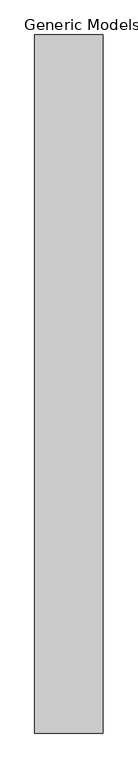
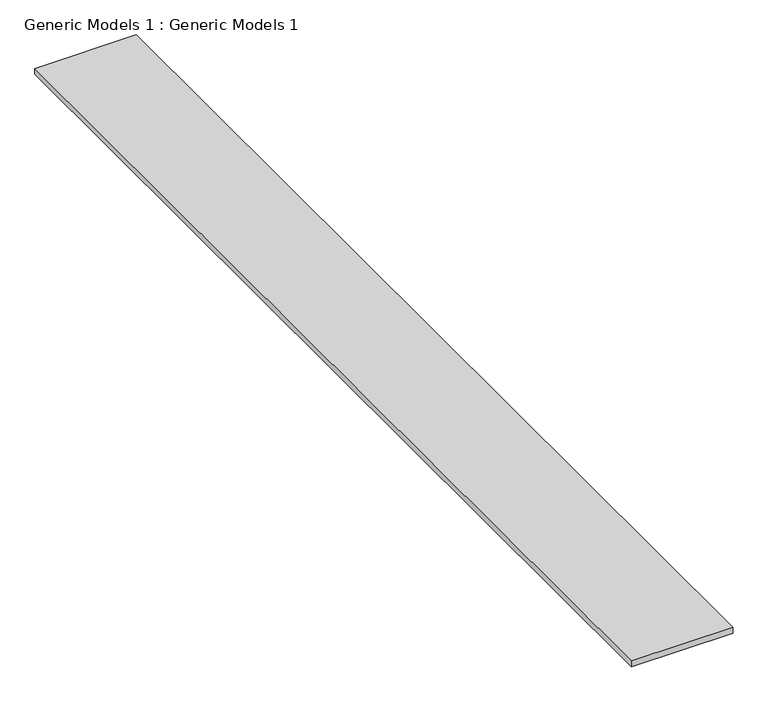
"""IFC4 building model written with IfcOpenShell, lengths in millimetres: proxy geometry, Generic Models 1 : Generic Models 1."""

from ifc_helpers import new_model, si_unit, frame, origin, place, context, project, spatial, polyline, outline, extrude, source, transform, mapped, element, save


def generic_models_1_generic_models_1_3256bdb4(model_context):
    return source(origin(), model_context, "Body", "SweptSolid", [
        extrude(outline(polyline([(10446.7316875, -460.7676788), (10446.7316875, 16989.0323212), (12161.0160983, 16989.0323212), (12161.0160983, -460.7676788), (10446.7316875, -460.7676788)])), frame((0.0, 0.0, -76.2), z_axis=(0.0, 0.0, 1.0), x_axis=(1.0, 0.0, 0.0)), (0.0, 0.0, 1.0), 104.242523),
    ])


if __name__ == "__main__":
    model = new_model("IFC4")
    model_context = context("Model", 3, world=origin())
    ifc_project = project(units=[si_unit("LENGTHUNIT", "METRE", prefix="MILLI")], contexts=[model_context])
    site = spatial("IfcSite", under=ifc_project)
    building = spatial("IfcBuilding", under=site)
    placement = place(None, origin())
    generic_models_1_generic_models_1_shape = generic_models_1_generic_models_1_3256bdb4(model_context)
    element("IfcBuildingElementProxy", 1, Name="Generic Models 1 : Generic Models 1", ObjectType="Generic Models 1 : Generic Models 1", at=placement, inside=building, context=model_context, shape_type="MappedRepresentation", body=[
        mapped(generic_models_1_generic_models_1_shape, transform((0.0, 0.0, 0.0), x_axis=(1.0, 0.0, 0.0), y_axis=(0.0, 1.0, 0.0), z_axis=(0.0, 0.0, 1.0))),
    ])
    save(model, "model.ifc")
